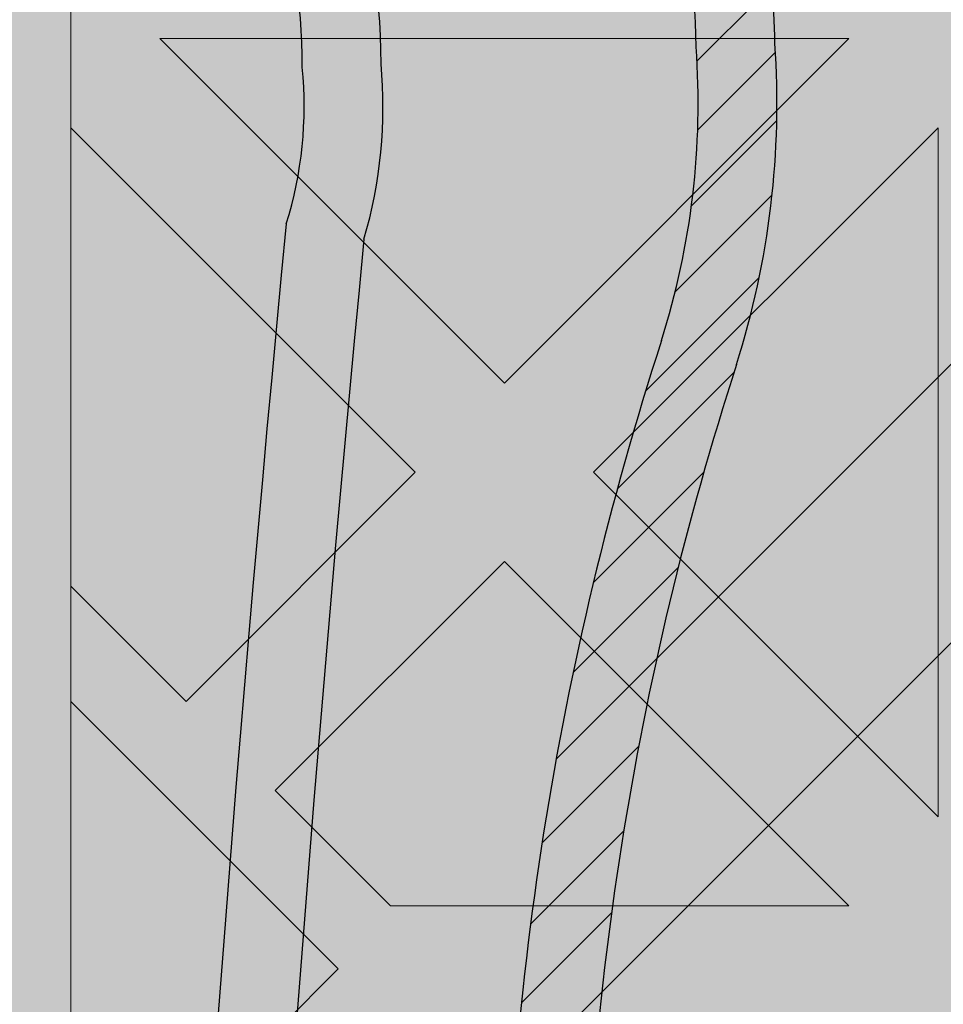
# Model space of a CAD drawing. Units: inches. Extents: x 844 to 2234, y 346 to 1084.
# Tile 17 of 93: x 1118.29 to 1120.159, y 701.25 to 703.242. Entities that reach past the tile are written whole.
import ezdxf

# ---------------------------------------------------------------- set-up
doc = ezdxf.new("R2010")
doc.units = ezdxf.units.IN
doc.header["$MEASUREMENT"] = 0
for name, color, linetype, lineweight in [('A-ANNO-DIMS', 2, 'Continuous', 18), ('furniture', 8, 'Continuous', 18), ('RA-AP-01$0$INT', 35, 'Continuous', 5)]:
    doc.layers.add(name, color=color, linetype=linetype, lineweight=lineweight)
doc.layers.add('RA-AP-01$0$FURN', color=3, linetype='Continuous')
doc.layers.add('RA-AP-01$0$WOOD', color=64, linetype='Continuous')
doc.styles.get("Standard").update_dxf_attribs({"font": 'arial.ttf'})
doc.dimstyles.get("Standard").update_dxf_attribs({"dimtxt": 6, "dimasz": 3, "dimexe": 0.18, "dimexo": 0.0625, "dimgap": 0.09, "dimtad": 0, "dimtih": 1, "dimtoh": 1, "dimdec": 1, "dimzin": 0, "dimdsep": 46, "dimlunit": 3, "dimtxsty": 'Standard', "dimblk": 'ARCHTICK', "dimcen": 0.09, "dimadec": 0, "dimazin": 0, "dimtfac": 1, "dimtdec": 1, "dimtofl": 0, "dimtmove": 0, "dimatfit": 3, "dimfxl": 1, "dimtolj": 1, "dimtzin": 0, "dimarcsym": 0})

# ---------------------------------------------------------------- blocks, each defined once
blk = doc.blocks.new('A$C18D01794')
at = {"layer": 'RA-AP-01$0$INT'}
blk.add_hatch(color=256, dxfattribs=at).paths.add_polyline_path([(4.505206456958071, -7.906712009588039), (5.305206456958072, -7.906712009588039), (5.305206456958072, -7.106712009588038), (5.255206456951893, -7.106712009588036), (5.25520645694868, -7.856712009570104), (4.555206456959269, -7.856712009588616), (4.555206456956052, -7.106712009588038), (4.505206456958073, -7.106712009588038)])
h = blk.add_hatch(color=256, dxfattribs=at)
h.paths.add_polyline_path([(4.585917135068448, -7.856712009587804), (4.614201406330596, -7.856712009587056), (4.668846067270487, -7.802067348644738), (4.723490728212344, -7.856712009584164), (4.771774999457151, -7.856712009582887), (4.826419660396886, -7.80206734864072), (4.862780050090322, -7.838427738332541), (4.844495778842715, -7.856712009580965), (4.862780050090411, -7.856712009580482), (4.905206456960182, -7.814285602707865), (4.947632863832445, -7.856712009578238), (4.965917135079675, -7.856712009577755), (4.947632863831759, -7.838427738330656), (4.983993253523576, -7.802067348637219), (5.038637914464627, -7.856712009575829), (5.08692218571208, -7.856712009574554), (5.141566846649976, -7.802067348634224), (5.196211507589851, -7.856712009571666), (5.224495778822615, -7.856712009570916), (4.905206456953975, -7.537422687702283)])
h.paths.add_polyline_path([(4.895206456956031, -7.575706958950402), (4.895206456958921, -7.684996280828174), (4.840561796018589, -7.630351619890275)], flags=16)
h.paths.add_polyline_path([(4.915206456955638, -7.575706958949956), (4.969851117895509, -7.630351619887399), (4.915206456957609, -7.684996280827732)], flags=16)
h.paths.add_polyline_path([(4.826419660395175, -7.644493755514321), (4.881064321335613, -7.699138416452331), (4.771774999456703, -7.69913841645522)], flags=16)
h.paths.add_polyline_path([(4.983993253519558, -7.644493755510815), (5.038637914460456, -7.699138416449285), (4.929348592581548, -7.69913841645126)], flags=16)
h.paths.add_polyline_path([(4.881064321336025, -7.719138416452334), (4.826419660397532, -7.773783077393256), (4.771774999457062, -7.719138416455217)], flags=16)
h.paths.add_polyline_path([(4.929348592582019, -7.71913841645126), (5.038637914460982, -7.719138416449284), (4.983993253522945, -7.773783077389749)], flags=16)
h.paths.add_polyline_path([(4.895206456960191, -7.733280552075633), (4.895206456962115, -7.806001331460164), (4.876922185715016, -7.824285602708492), (4.840561796021581, -7.787925213016675)], flags=16)
h.paths.add_polyline_path([(4.915206456958487, -7.733280552075187), (4.969851117899527, -7.787925213013798), (4.933490728206909, -7.824285602708034), (4.9152064569598, -7.806001331461736)], flags=16)
h.paths.add_polyline_path([(4.757632863832376, -7.733280552079264), (4.812277524772842, -7.787925213017304), (4.757632863834348, -7.842569873958233)], flags=16)
h.paths.add_polyline_path([(4.737632863832376, -7.73328055207979), (4.737632863834348, -7.842569873958701), (4.682988202893906, -7.787925213020692)], flags=16)
h.paths.add_polyline_path([(5.05278005008503, -7.733280552072701), (5.052780050087917, -7.842569873951664), (4.998135389146995, -7.787925213013169)], flags=16)
h.paths.add_polyline_path([(5.072780050085024, -7.733280552072333), (5.127424711025931, -7.787925213010806), (5.072780050087916, -7.842569873951244)], flags=16)
h.paths.add_polyline_path([(4.935917135072783, -7.506712009583784), (5.255206456948811, -7.826001331459767), (5.255206456948932, -7.797717060211899), (5.200561796010279, -7.743072399273238), (5.255206456949403, -7.688427738334128), (5.25520645694961, -7.640143467086677), (5.200561796009787, -7.585498806146837), (5.236922185702417, -7.549138416454212), (5.255206456949919, -7.56742268770172), (5.255206456949998, -7.549138416454178), (5.212780050078687, -7.506712009583814), (5.25520645695036, -7.464285602712145), (5.255206456950438, -7.446001331464763), (5.236922185702424, -7.464285602712779), (5.200561796009796, -7.427925213020149), (5.255206456950753, -7.373280552079203), (5.25520645695096, -7.324996280834394), (5.200561796010322, -7.270351619893748), (5.255206456951428, -7.215706958952649), (5.255206456951547, -7.187422687705071)])
h.paths.add_polyline_path([(5.042988202883395, -7.42792521302065), (5.097632863823085, -7.373280552080975), (5.097632863822622, -7.482569873959883)], flags=16)
h.paths.add_polyline_path([(5.028846067259663, -7.442067348644384), (5.083490728198774, -7.496712009583504), (4.974201406321001, -7.496712009583035)], flags=16)
h.paths.add_polyline_path([(5.117632863823087, -7.37328055208089), (5.172277524762331, -7.42792521302015), (5.11763286382262, -7.482569873959851)], flags=16)
h.paths.add_polyline_path([(5.08349072819877, -7.516712009582191), (5.028846067259652, -7.571356670521302), (4.974201406320998, -7.516712009582638)], flags=16)
h.paths.add_polyline_path([(5.131774999446817, -7.35913841645716), (5.186419660386065, -7.413783077396415), (5.241064321325782, -7.359138416456712)], flags=17)
h.paths.add_polyline_path([(5.131774999446228, -7.496712009583703), (5.186419660386065, -7.442067348643883), (5.222780050079488, -7.478427738337313), (5.204495778832781, -7.496712009584014)], flags=16)
h.paths.add_polyline_path([(5.097632863822613, -7.530854145205813), (5.097632863823061, -7.640143467084723), (5.042988202883383, -7.585498806145032)], flags=16)
h.paths.add_polyline_path([(5.131774999446899, -7.339138416457162), (5.241064321325809, -7.339138416456712), (5.186419660386591, -7.284493755517479)], flags=17)
h.paths.add_polyline_path([(5.131774999446226, -7.516712009581999), (5.204495778830767, -7.516712009581702), (5.22278005007868, -7.534996280829206), (5.186419660386049, -7.571356670521828)], flags=16)
h.paths.add_polyline_path([(5.11763286382262, -7.530854145205852), (5.17227752476232, -7.585498806145562), (5.117632863823064, -7.64014346708481)], flags=16)
h.paths.add_polyline_path([(5.186419660386069, -7.599640941770585), (5.241064321325754, -7.654285602710281), (5.131774999446791, -7.654285602709814)], flags=16)
h.paths.add_polyline_path([(5.131774999446872, -7.674285602709813), (5.24106432132578, -7.674285602710282), (5.186419660386554, -7.728930263649504)], flags=16)
h.paths.add_polyline_path([(5.255206456951811, -7.126001331467467), (5.255206456951895, -7.106712009588038), (4.555206456956052, -7.106712009588038), (4.555206456956136, -7.12600133146746), (4.905206456953973, -7.476001331465289)])
h.paths.add_polyline_path([(4.983993253513404, -7.368930263651977), (4.92934859257295, -7.314285602713969), (5.03863791445186, -7.314285602711063)], flags=16)
h.paths.add_polyline_path([(4.969851117889988, -7.383072399276016), (4.915206456952556, -7.437717060215906), (4.915206456949648, -7.328427738338133)], flags=16)
h.paths.add_polyline_path([(4.929348592572535, -7.294285602713971), (4.983993253511019, -7.239640941773039), (5.038637914451496, -7.294285602711065)], flags=16)
h.paths.add_polyline_path([(5.052780050074912, -7.280143467087016), (4.998135389134438, -7.225498806148989), (5.052780050072919, -7.170854145208052)], flags=16)
h.paths.add_polyline_path([(5.07278005007491, -7.280143467086489), (5.072780050072918, -7.170854145207579), (5.127424711013374, -7.225498806145578)], flags=16)
h.paths.add_polyline_path([(4.89520645695295, -7.437717060216355), (4.840561796013067, -7.383072399278919), (4.895206456950961, -7.328427738338582)], flags=16)
h.paths.add_polyline_path([(4.915206456948365, -7.280143467090674), (4.915206456946434, -7.207422687704125), (4.933490728192729, -7.18913841645701), (4.969851117886972, -7.225498806149623)], flags=16)
h.paths.add_polyline_path([(4.881064321327021, -7.314285602715054), (4.82641966038902, -7.368930263655506), (4.771774999448108, -7.314285602717047)], flags=16)
h.paths.add_polyline_path([(4.895206456950073, -7.280143467091125), (4.840561796009022, -7.225498806152518), (4.876922185700835, -7.18913841645908), (4.895206456948749, -7.207422687706589)], flags=16)
h.paths.add_polyline_path([(4.983993253510392, -7.211356670525576), (4.947632863816944, -7.174996280833758), (4.965917135064043, -7.156712009585847), (5.038637914448995, -7.156712009584522)], flags=16)
h.paths.add_polyline_path([(4.881064321326543, -7.294285602715056), (4.771774999447578, -7.294285602717046), (4.826419660385607, -7.239640941776569)], flags=16)
h.paths.add_polyline_path([(4.905206456946447, -7.19913841645844), (4.862780050074785, -7.156712009587725), (4.947632863816685, -7.156712009586302)], flags=16)
h.paths.add_polyline_path([(5.14156684663679, -7.211356670521528), (5.086922185696452, -7.156712009583639), (5.196211507574223, -7.156712009581651)], flags=16)
h.paths.add_polyline_path([(4.8264196603837, -7.211356670529104), (4.771774999442643, -7.156712009590501), (4.8444957788276, -7.156712009588568), (4.862780050075511, -7.17499628083566)], flags=16)
h.paths.add_polyline_path([(4.812277524760289, -7.225498806153156), (4.757632863822258, -7.28014346709363), (4.757632863819352, -7.170854145214669)], flags=16)
h.paths.add_polyline_path([(4.73763286382226, -7.280143467093997), (4.682988202881349, -7.22549880615554), (4.737632863819352, -7.170854145215086)], flags=16)
h.paths.add_polyline_path([(4.723490728195188, -7.156712009591787), (4.668846067257299, -7.211356670532127), (4.614201406317417, -7.156712009594693)], flags=16)
h.paths.add_polyline_path([(4.597632863829262, -7.506712009583814), (4.555206456957951, -7.54913841645418), (4.555206456958029, -7.56742268770172), (4.573490728205535, -7.549138416454212), (4.609851117898167, -7.585498806146839), (4.555206456958338, -7.640143467086675), (4.555206456958546, -7.688427738334125), (4.60985111789767, -7.743072399273238), (4.555206456959015, -7.797717060211899), (4.555206456959138, -7.826001331459767), (4.874495778835167, -7.506712009583786), (4.5552064569564, -7.187422687705062), (4.555206456956523, -7.215706958952644), (4.609851117897629, -7.270351619893746), (4.555206456956988, -7.324996280834396), (4.555206456957198, -7.373280552079195), (4.609851117898153, -7.427925213020147), (4.573490728205528, -7.464285602712779), (4.555206456957507, -7.446001331464756), (4.555206456957585, -7.464285602712143)])
h.paths.add_polyline_path([(4.712780050085332, -7.482569873959882), (4.712780050084863, -7.373280552080972), (4.767424711024555, -7.42792521302065)], flags=16)
h.paths.add_polyline_path([(4.726922185709173, -7.496712009583504), (4.781566846648288, -7.442067348644384), (4.836211507586949, -7.496712009583033)], flags=16)
h.paths.add_polyline_path([(4.692780050085327, -7.482569873959851), (4.638135389145619, -7.427925213020149), (4.692780050084865, -7.373280552080892)], flags=16)
h.paths.add_polyline_path([(4.726922185709182, -7.516712009582191), (4.836211507586949, -7.51671200958264), (4.7815668466483, -7.571356670521304)], flags=16)
h.paths.add_polyline_path([(4.678637914461726, -7.496712009583706), (4.605917135075169, -7.496712009584014), (4.587632863828464, -7.478427738337311), (4.623993253521887, -7.442067348643881)], flags=16)
h.paths.add_polyline_path([(4.712780050085336, -7.530854145205816), (4.767424711024568, -7.585498806145034), (4.71278005008489, -7.640143467084724)], flags=16)
h.paths.add_polyline_path([(4.678637914461726, -7.516712009582001), (4.623993253521899, -7.571356670521829), (4.587632863829271, -7.534996280829206), (4.605917135077185, -7.5167120095817)], flags=16)
h.paths.add_polyline_path([(4.692780050085336, -7.530854145205848), (4.692780050084889, -7.64014346708481), (4.638135389145632, -7.585498806145562)], flags=16)
h.paths.add_polyline_path([(4.623993253521885, -7.413783077396415), (4.678637914461131, -7.359138416457161), (4.56934859258217, -7.359138416456712)], flags=17)
h.paths.add_polyline_path([(4.623993253521901, -7.599640941770568), (4.678637914461158, -7.654285602709814), (4.569348592582195, -7.654285602710281)], flags=16)
h.paths.add_polyline_path([(4.678637914461051, -7.339138416457162), (4.623993253521361, -7.284493755517479), (4.569348592582143, -7.339138416456712)], flags=17)
h.paths.add_polyline_path([(4.678637914461076, -7.674285602709813), (4.623993253521399, -7.728930263649504), (4.569348592582167, -7.674285602710281)], flags=16)
h = blk.add_hatch(color=256, dxfattribs=at)
h.paths.add_polyline_path([(4.781566846647504, -7.442067348645805), (4.836211507586161, -7.496712009584463), (4.726922185708388, -7.496712009584918)])
h.paths.add_polyline_path([(4.836211507586161, -7.516712009584068), (4.781566846647504, -7.571356670522723), (4.726922185708388, -7.516712009583606)])
h.paths.add_polyline_path([(4.76742471102377, -7.585498806146453), (4.712780050084083, -7.640143467086137), (4.712780050084542, -7.530854145207227)])
h.paths.add_polyline_path([(4.692780050084544, -7.530854145207257), (4.692780050084084, -7.64014346708622), (4.638135389144834, -7.585498806146965)])
h.paths.add_polyline_path([(4.678637914460932, -7.516712009583407), (4.623993253521102, -7.571356670523233), (4.587632863827676, -7.53499628082981), (4.605917135074382, -7.516712009583104)])
h.paths.add_polyline_path([(4.573490728204743, -7.54913841645434), (4.60985111789737, -7.585498806146969), (4.555206456957541, -7.640143467086797), (4.555206456957237, -7.567422687701846)])
h.paths.add_polyline_path([(4.623993253521098, -7.599640941770699), (4.67863791446035, -7.654285602709951), (4.56934859258139, -7.654285602710407)])
h.paths.add_polyline_path([(4.678637914460275, -7.67428560270995), (4.623993253520583, -7.728930263649637), (4.56934859258136, -7.674285602710405)])
h.paths.add_polyline_path([(4.609851117896854, -7.743072399273369), (4.555206456958196, -7.797717060212026), (4.555206456957738, -7.688427738334254)])
h.paths.add_polyline_path([(4.597632863828475, -7.506712009583301), (4.555206456957283, -7.549138416454495), (4.555206456956805, -7.464285602712587)])
h.paths.add_polyline_path([(4.678637914460932, -7.496712009585113), (4.605917135076396, -7.496712009585417), (4.587632863828479, -7.478427738337913), (4.623993253521104, -7.442067348645284)])
h.paths.add_polyline_path([(4.692780050084091, -7.373280552082301), (4.692780050084548, -7.482569873961267), (4.638135389144834, -7.427925213021552)])
h.paths.add_polyline_path([(4.767424711023772, -7.427925213022072), (4.712780050084545, -7.48256987396129), (4.712780050084089, -7.373280552082384)])
h.paths.add_polyline_path([(4.67863791446036, -7.359138416457298), (4.623993253521105, -7.41378307739655), (4.569348592581399, -7.35913841645684)])
h.paths.add_polyline_path([(4.609851117897371, -7.427925213020278), (4.573490728204743, -7.464285602712907), (4.555206456957237, -7.446001331465401), (4.555206456957548, -7.373280552080448)])
h.paths.add_polyline_path([(4.623993253520596, -7.284493755517612), (4.67863791446028, -7.339138416457299), (4.569348592581367, -7.339138416456838)])
h.paths.add_polyline_path([(4.609851117896867, -7.270351619893878), (4.555206456957749, -7.324996280832994), (4.55520645695821, -7.21570695895522)])
for p, q in [((4.555206456956052, -7.106712009588036), (4.555206456959269, -7.856712009588616)), ((4.597632863829264, -7.506712009583814), (4.55520645695807, -7.464285602712626)), ((4.55520645695807, -7.464285602712626), (4.555206456957598, -7.549138416454534)), ((4.597632863829264, -7.506712009583814), (4.555206456957598, -7.549138416454534)), ((4.605917135074869, -7.516712009584017), (4.587632863829269, -7.534996280829206)), ((4.605917135076771, -7.5167120095817), (4.678637914461723, -7.516712009581999)), ((4.678637914461723, -7.516712009581999), (4.623993253521898, -7.571356670521829)), ((4.692780050085336, -7.530854145205847), (4.638135389145632, -7.585498806145562)), ((4.692780050084889, -7.64014346708481), (4.692780050085336, -7.530854145205847)), ((4.623993253521899, -7.571356670521829), (4.587632863829269, -7.534996280829206)), ((4.555206456958031, -7.56742268770172), (4.573490728205535, -7.549138416454212)), ((4.609851117898167, -7.585498806146839), (4.573490728205535, -7.549138416454214)), ((4.555206456958033, -7.56742268770172), (4.555206456958345, -7.640143467086671)), ((4.555206456958345, -7.640143467086671), (4.609851117898167, -7.585498806146837)), ((4.692780050084889, -7.64014346708481), (4.638135389145632, -7.585498806145562)), ((4.569348592582195, -7.654285602710281), (4.623993253521901, -7.599640941770568)), ((4.678637914461158, -7.654285602709814), (4.623993253521901, -7.599640941770568)), ((4.678637914461158, -7.654285602709814), (4.569348592582195, -7.654285602710281))]:
    blk.add_line(p, q, dxfattribs=at)
blk = doc.blocks.new('A$C32926AE1')
at = {"layer": 'RA-AP-01$0$WOOD'}
h = blk.add_hatch(color=256, dxfattribs=at)
h.dxf.hatch_style = 1
h.paths.add_polyline_path([(5.157430609644524, 4.573483066760929, -0.1009492694046607), (5.155401577623758, 4.593365984175333, -0.1842662638101597), (5.172249623284174, 4.638795604568598, 0.2056608120311276), (5.179560981299304, 4.661316324430096, 0.3614336704623542), (5.134352340494423, 4.706524965234944, 0.2056608120311297), (5.111831620632933, 4.699213607219793, -0.1842662638101113), (5.066402000239693, 4.682365561559342, -0.1055311479399994), (5.045656153913092, 4.68467289944697, 0.1567636581983829), (4.763886414745334, 4.684672899446966, -0.1055311479399895), (4.743140568418733, 4.68236556155934, -0.1842662638100833), (4.6977109480255, 4.69921360721979, 0.2056608120302612), (4.675190228164109, 4.706524965234949, 0.3614336704708441), (4.629981587358889, 4.66131632442871, 0.2056608120245944), (4.637292945374126, 4.638795604567974, -0.1842662638101024), (4.654140991034615, 4.59336598417475, -0.1009492694055169), (4.652111959013835, 4.573483066760181, 0.021410119221476), (4.629748025606143, 4.156712009541676, 0.0214101192214795), (4.652111959013809, 3.739940952323101, -0.1009492694059586), (4.654140991034615, 3.720058034908448, -0.1842662638100975), (4.637292945374126, 3.674628414515226, 0.2056608120245705), (4.629981587358889, 3.652107694654492, 0.3614336704708879), (4.675190228164113, 3.606899053848249, 0.2056608120302384), (4.697710948025501, 3.614210411863408, -0.1842662638100995), (4.743140568418738, 3.63105845752386, -0.1055311479402541), (4.763886414745388, 3.628751119636215, 0.1567636581983776), (5.045656153913137, 3.628751119636244, -0.1055311479397538), (5.066402000239692, 3.631058457523857, -0.1842662638101067), (5.111831620632931, 3.614210411863407, 0.2056608120310924), (5.134352340494417, 3.606899053848256, 0.3614336704624001), (5.179560981299307, 3.652107694653103, 0.2056608120311314), (5.172249623284175, 3.6746284145146, -0.1842662638101402), (5.155401577623758, 3.72005803490786, -0.1009492694051366), (5.15743060964455, 3.739940952322354, 0.0214101192215073), (5.179794543052287, 4.156712009541468, 0.0214101192215252)])
h.paths.add_polyline_path([(4.639748609479751, 4.156712009541513, 0.0213537860821624), (4.661970494867118, 3.741887061152232, -0.094075836301374), (4.664143710413708, 3.7196126951003, -0.1824818158568985), (4.644813765429836, 3.668037719127816, 0.2056608120245319), (4.639939526753007, 3.653023905887301, 0.3614336704710246), (4.676106439397173, 3.616856993242342, 0.2056608120302234), (4.691120252638095, 3.621731231919122, -0.1824818158602558), (4.742695228611606, 3.641061176902986, -0.1029891339458722), (4.766991894714349, 3.638256818950944, 0.156709409989566), (5.042550673941472, 3.638256818950105, -0.102989133958497), (5.066847340047078, 3.641061176902949, -0.1824818158594995), (5.118422316020358, 3.621731231919103, 0.2056608120311416), (5.133436129261316, 3.616856993242346, 0.3614336704621468), (5.169603041905217, 3.653023905886178, 0.2056608120310986), (5.164728803228477, 3.668037719127177, -0.1824818158565612), (5.145398858244737, 3.719612695099578, -0.0940758363009313), (5.147572073791232, 3.741887061151398, 0.0213537860822023), (5.169793959178681, 4.156712009541451, 0.0213537860822226), (5.147572073791203, 4.571536957931898, -0.0940758363005034), (5.145398858244737, 4.59381132398362, -0.1824818158565587), (5.164728803228476, 4.645386299956021, 0.2056608120311045), (5.169603041905216, 4.66040011319702, 0.3614336704621845), (5.133436129261313, 4.696567025840856, 0.2056608120310773), (5.118422316020359, 4.691692787164098, -0.182481815859508), (5.066847340047078, 4.67236284218025, -0.1029891339584606), (5.04255067394148, 4.675167200133092, 0.156709409989566), (4.766991894714357, 4.675167200132257, -0.1029891339458842), (4.742695228611611, 4.672362842180213, -0.1824818158602725), (4.691120252638095, 4.691692787164077, 0.2056608120302152), (4.676106439397174, 4.696567025840858, 0.3614336704710363), (4.639939526753005, 4.660400113195899, 0.2056608120245495), (4.644813765429837, 4.645386299955384, -0.1824818158568934), (4.664143710413708, 4.593811323982902, -0.0940758363009187), (4.661970494867149, 4.571536957931074, 0.021353786082177)], flags=16)
h.paths.add_polyline_path([(5.129794543052235, 4.432167055276933, -0.0141661062790638), (5.130152669293814, 4.156927903047693, -0.0141661062790647), (5.129794543052234, 3.881688750818433, -0.0785247771143638), (5.10979738006795, 3.755143611847103, 0.0945969212073497), (5.105408519571111, 3.717898134952927, 0.1043170707844957), (5.116074640131521, 3.670385395016088, 0.1043170707864965), (5.068561900193738, 3.681051515576561, 0.09459692119553), (5.031316423304057, 3.676662655080835, -0.1580239521427272), (4.778226145355827, 3.676662655080367, 0.0945969211986668), (4.740980668464973, 3.681051515576592, 0.1043170707882822), (4.693467928526415, 3.670385395015844, 0.1043170707867916), (4.704134049087309, 3.717898134953662, 0.0945969211972894), (4.69974518859162, 3.755143611844042, -0.0785247771163196), (4.679748025606343, 3.881688750818406, -0.0141661062790663), (4.679389899364763, 4.156927903047693, -0.0141661062790672), (4.679748025606343, 4.432167055276998, -0.0785247771163064), (4.699745188591625, 4.55871219425134, 0.094596921197333), (4.704134049087308, 4.595957671141738, 0.1043170707867205), (4.693467928526416, 4.643470411079523, 0.1043170707882628), (4.740980668464965, 4.632804290518776, 0.0945969211988114), (4.778226145355874, 4.637193151015016, -0.158023952142669), (5.031316423304015, 4.637193151014546, 0.0945969211956361), (5.068561900193736, 4.632804290518806, 0.1043170707864979), (5.11607464013152, 4.643470411079278, 0.1043170707844617), (5.105408519571112, 4.595957671142455, 0.0945969212074597), (5.109797380067959, 4.558712194248236, -0.0785247771143467)], flags=0)
h.paths.add_polyline_path([(5.119794532311105, 4.432259799204851, -0.0142000800617244), (5.120156169157484, 4.156927903047701, -0.0142000800617277), (5.119794532311105, 3.881596006890482, -0.0784894509520253), (5.100273383573699, 3.758192358677797, 0.0940138827242913), (5.095413455884425, 3.717477693979438, 0.0606271852308753), (5.099615656341024, 3.686844378806616, 0.0606271852322524), (5.068982341167493, 3.691046579263239, 0.0940138827010453), (5.028267676478798, 3.686186651576848, -0.1580706864508061), (4.781274892180912, 3.686186651576435, 0.0940138827026903), (4.740560227491556, 3.691046579263279, 0.0606271852339895), (4.709926912317155, 3.686844378806508, 0.0606271852329405), (4.714129112773991, 3.717477693980356, 0.094013882701304), (4.709269185087677, 3.758192358669163, -0.0784894509577193), (4.689748036347473, 3.881596006890469, -0.014200080061729), (4.689386399501094, 4.156927903047709, -0.0142000800617217), (4.689748036347473, 4.432259799204808, -0.078489450957724), (4.709269185087651, 4.555663447426125, 0.0940138827014585), (4.714129112773992, 4.596378112114996, 0.0606271852329731), (4.709926912317154, 4.62701142728886, 0.0606271852340196), (4.74056022749157, 4.622809226832087, 0.0940138827024997), (4.781274892180847, 4.627669154518912, -0.1580706864508359), (5.028267676478777, 4.627669154518526, 0.0940138827010946), (5.068982341167492, 4.622809226832129, 0.060627185232254), (5.099615656341024, 4.627011427288751, 0.0606271852308727), (5.095413455884425, 4.59637811211593, 0.0940138827241088), (5.100273383573675, 4.555663447417647, -0.0784894509520978)], flags=0)
h.paths.add_polyline_path([(5.06978912287499, 4.430218106756144, -0.014241683694547), (5.070173729147532, 4.156927903047672, -0.0142416836945458), (5.06978912287499, 3.883637699339223, -0.0800609523125196), (5.052662118612511, 3.773463122773442, 0.0526421978001116), (5.04590916754064, 3.740550867606997, 0.0526421977992423), (5.012996912374707, 3.73379791653534, -0.1583028414718258), (4.796545656286308, 3.73379791653451, 0.0526421978034211), (4.763633401117837, 3.740550867607021, 0.0526421978018622), (4.756880450045755, 3.773463122774558, -0.0800609523117106), (4.739753445783639, 3.883637699339268, -0.0142416836945435), (4.739368839511098, 4.156927903047671, -0.0142416836945477), (4.739753445783639, 4.430218106756155, -0.0800609523116345), (4.75688045004574, 4.540392683320762, 0.052642197801941), (4.763633401117837, 4.573304938488346, 0.0526421978035071), (4.796545656286361, 4.580057889560873, -0.1583028414717561), (5.012996912374669, 4.580057889560039, 0.0526421977993048), (5.04590916754064, 4.57330493848837, 0.0526421978002057), (5.052662118612529, 4.540392683321868, -0.080060952312477)], flags=0)
h.paths.add_polyline_path([(5.049789715110557, 4.43038092723357, -0.0143097550741839), (5.05018085590259, 4.156927903047715, -0.0143097550741854), (5.049789715110558, 3.883474878861827, -0.0800685599149176), (5.03362098255317, 3.779581877367999, 0.0306258898956367), (5.028241146483733, 3.758218888663947, 0.0306258898977031), (5.006878157778253, 3.75283905259408, -0.1583983521624096), (4.802664410878162, 3.752839052594731, 0.0306258898946014), (4.781301422174808, 3.758218888663924, 0.0306258898967912), (4.775921586105202, 3.779581877368794, -0.080068559914251), (4.759752853548071, 3.883474878861786, -0.0143097550741854), (4.759361712756037, 4.156927903047671, -0.0143097550741854), (4.759752853548071, 4.430380927233557, -0.0800685599142479), (4.775921586105193, 4.534273928726546, 0.0306258898968306), (4.781301422174808, 4.555636917431444, 0.0306258898945754), (4.802664410878143, 4.561016753500631, -0.1583983521624168), (5.006878157778244, 4.561016753501291, 0.0306258898977177), (5.028241146483733, 4.555636917431421, 0.0306258898958182), (5.03362098255321, 4.534273928727244, -0.080068559914796)], flags=0)
h.paths.add_polyline_path([(4.999766070382627, 4.428171244713864, -0.0143443147609634), (5.000198441819402, 4.156927903047689, -0.0143443147609612), (4.999766070382627, 3.885684561381556, -0.0784641635803329), (4.987356730658798, 3.799103304488872, -0.1506053783831347), (4.822185837999821, 3.79910330448882, -0.0784641635803318), (4.809776498276007, 3.885684561381509, -0.014344314760963), (4.809344126839227, 4.156927903047677, -0.0143443147609645), (4.809776498276007, 4.428171244713873, -0.0784641635803192), (4.822185837999822, 4.514752501606549, -0.1506053783831338), (4.987356730658798, 4.514752501606494, -0.078464163580285)], flags=0)
h.paths.add_polyline_path([(4.979755254238824, 4.42764379880488, -0.0143772539198268), (4.980205517789977, 4.156927903047693, -0.0143772539198275), (4.979755254238824, 3.886212007290489, -0.0689242507424422), (4.971183264704897, 3.815276770442801, -0.1296645318904179), (4.838359303953726, 3.815276770442746, -0.0689242507424186), (4.829787314419809, 3.886212007290419, -0.0143772539198292), (4.829337050868653, 4.156927903047653, -0.0143772539198325), (4.829787314419809, 4.427643798804946, -0.0689242507424211), (4.838359303953725, 4.498579035652621, -0.1296645318904187), (4.971183264704897, 4.498579035652565, -0.0689242507424401)], flags=0)
h = blk.add_hatch(color=256, dxfattribs=at)
h.dxf.hatch_style = 1
h.paths.add_polyline_path([(5.145398858244737, 4.59381132398362, -0.1824818158565616), (5.164728803228476, 4.645386299956021, 0.2056608120311045), (5.169603041905216, 4.66040011319702, 0.3614336704621845), (5.133436129261313, 4.696567025840856, 0.2056608120310773), (5.118422316020359, 4.691692787164098, -0.182481815859508), (5.066847340047078, 4.67236284218025, -0.1029891339584606), (5.04255067394148, 4.675167200133092, 0.156709409989566), (4.766991894714357, 4.675167200132257, -0.1029891339458842), (4.742695228611611, 4.672362842180213, -0.1824818158602725), (4.691120252638095, 4.691692787164077, 0.2056608120302152), (4.676106439397174, 4.696567025840858, 0.3614336704710363), (4.639939526753005, 4.660400113195899, 0.2056608120245495), (4.644813765429837, 4.645386299955384, -0.1824818158568934), (4.664143710413708, 4.593811323982902, -0.0940758363009187), (4.661970494867149, 4.571536957931074, 0.0213537860821772), (4.639748609479751, 4.156712009541507, 0.0213537860821625), (4.661970494867119, 3.741887061152226, -0.0940758363013071), (4.664143710413708, 3.719612695100309, -0.1824818158569294), (4.644813765429836, 3.668037719127816, 0.2056608120245319), (4.639939526753007, 3.653023905887301, 0.3614336704710246), (4.676106439397173, 3.616856993242342, 0.2056608120302234), (4.691120252638095, 3.621731231919122, -0.1824818158602558), (4.742695228611606, 3.641061176902986, -0.1029891339458722), (4.766991894714349, 3.638256818950944, 0.156709409989566), (5.042550673941472, 3.638256818950105, -0.102989133958497), (5.066847340047078, 3.641061176902949, -0.1824818158594995), (5.118422316020358, 3.621731231919103, 0.2056608120311416), (5.133436129261316, 3.616856993242346, 0.3614336704621468), (5.169603041905217, 3.653023905886178, 0.2056608120310986), (5.164728803228477, 3.668037719127177, -0.1824818158565612), (5.145398858244737, 3.719612695099578, -0.0940758363009313), (5.147572073791232, 3.741887061151398, 0.0213537860822023), (5.169793959178681, 4.156712009541451, 0.0213537860822226), (5.147572073791203, 4.571536957931898, -0.0940758363004996)])
h.paths.add_polyline_path([(5.109797380067958, 4.55871219424824, -0.0785247771143472), (5.129794543052234, 4.432167055276936, -0.0141661062790644), (5.130152669293814, 4.156927903047685, -0.014166106279066), (5.129794543052234, 3.881688750818401, -0.0785247771143517), (5.109797380067946, 3.755143611847092, 0.0945969212073132), (5.105408519571111, 3.717898134952929, 0.1043170707844995), (5.116074640131521, 3.670385395016088, 0.1043170707864965), (5.068561900193738, 3.681051515576561, 0.09459692119553), (5.031316423304057, 3.676662655080835, -0.1580239521427272), (4.778226145355827, 3.676662655080367, 0.0945969211986668), (4.740980668464973, 3.681051515576592, 0.1043170707882822), (4.693467928526415, 3.670385395015844, 0.1043170707867916), (4.704134049087309, 3.717898134953662, 0.0945969211972894), (4.69974518859162, 3.755143611844042, -0.0785247771163196), (4.679748025606343, 3.881688750818406, -0.0141661062790663), (4.679389899364763, 4.156927903047693, -0.0141661062790672), (4.679748025606343, 4.432167055276998, -0.0785247771163064), (4.699745188591625, 4.55871219425134, 0.094596921197333), (4.704134049087308, 4.595957671141738, 0.1043170707867205), (4.693467928526416, 4.643470411079523, 0.1043170707882628), (4.740980668464965, 4.632804290518776, 0.0945969211988114), (4.778226145355874, 4.637193151015016, -0.158023952142669), (5.031316423304015, 4.637193151014546, 0.0945969211956361), (5.068561900193736, 4.632804290518806, 0.1043170707864979), (5.11607464013152, 4.643470411079278, 0.1043170707844617), (5.105408519571112, 4.595957671142455, 0.0945969212074504)], flags=16)
h.paths.add_polyline_path([(5.100273383573655, 4.55566344741771, -0.0784894509521388), (5.119794532311105, 4.432259799204852, -0.0142000800617252), (5.120156169157484, 4.156927903047686, -0.014200080061726), (5.119794532311105, 3.881596006890502, -0.0784894509520446), (5.100273383573696, 3.758192358677786, 0.0940138827242721), (5.095413455884425, 3.717477693979436, 0.0606271852308692), (5.099615656341024, 3.686844378806616, 0.0606271852322522), (5.068982341167493, 3.691046579263239, 0.0940138827010453), (5.028267676478798, 3.686186651576848, -0.1580706864508061), (4.781274892180912, 3.686186651576435, 0.0940138827026903), (4.740560227491556, 3.691046579263279, 0.0606271852339895), (4.709926912317155, 3.686844378806508, 0.0606271852329405), (4.714129112773991, 3.717477693980356, 0.094013882701304), (4.709269185087677, 3.758192358669163, -0.0784894509577193), (4.689748036347473, 3.881596006890469, -0.014200080061729), (4.689386399501094, 4.156927903047709, -0.0142000800617217), (4.689748036347473, 4.432259799204808, -0.078489450957724), (4.709269185087651, 4.555663447426125, 0.0940138827014585), (4.714129112773992, 4.596378112114996, 0.0606271852329731), (4.709926912317154, 4.62701142728886, 0.0606271852340196), (4.74056022749157, 4.622809226832087, 0.0940138827024997), (4.781274892180847, 4.627669154518912, -0.1580706864508359), (5.028267676478777, 4.627669154518526, 0.0940138827010946), (5.068982341167492, 4.622809226832129, 0.060627185232254), (5.099615656341024, 4.627011427288751, 0.0606271852308727), (5.095413455884425, 4.59637811211593, 0.094013882723957)], flags=0)
h.paths.add_polyline_path([(5.04590916754064, 4.57330493848837, 0.0526421978002057), (5.052662118612529, 4.540392683321868, -0.0800609523124783), (5.06978912287499, 4.430218106756142, -0.0142416836945469), (5.070173729147532, 4.156927903047672, -0.0142416836945458), (5.06978912287499, 3.883637699339223, -0.0800609523125196), (5.052662118612511, 3.773463122773442, 0.0526421978001116), (5.04590916754064, 3.740550867606997, 0.0526421977992423), (5.012996912374707, 3.73379791653534, -0.1583028414718258), (4.796545656286308, 3.73379791653451, 0.0526421978034211), (4.763633401117837, 3.740550867607021, 0.0526421978018622), (4.756880450045755, 3.773463122774558, -0.0800609523117106), (4.739753445783639, 3.883637699339268, -0.0142416836945435), (4.739368839511098, 4.156927903047671, -0.0142416836945477), (4.739753445783639, 4.430218106756155, -0.0800609523116345), (4.75688045004574, 4.540392683320762, 0.052642197801941), (4.763633401117837, 4.573304938488346, 0.0526421978035071), (4.796545656286361, 4.580057889560873, -0.1583028414717561), (5.012996912374669, 4.580057889560039, 0.0526421977993048)], flags=0)
h.paths.add_polyline_path([(5.028241146483733, 4.555636917431422, 0.0306258898956949), (5.033620982553182, 4.534273928727329, -0.0800685599148649), (5.049789715110557, 4.430380927233569, -0.0143097550741839), (5.05018085590259, 4.156927903047715, -0.0143097550741854), (5.049789715110558, 3.883474878861827, -0.0800685599149176), (5.03362098255317, 3.779581877367999, 0.0306258898956367), (5.028241146483733, 3.758218888663947, 0.0306258898977031), (5.006878157778253, 3.75283905259408, -0.1583983521624096), (4.802664410878162, 3.752839052594731, 0.0306258898946014), (4.781301422174808, 3.758218888663924, 0.0306258898967912), (4.775921586105202, 3.779581877368794, -0.080068559914251), (4.759752853548071, 3.883474878861786, -0.0143097550741854), (4.759361712756037, 4.156927903047671, -0.0143097550741854), (4.759752853548071, 4.430380927233557, -0.0800685599142479), (4.775921586105193, 4.534273928726546, 0.0306258898968306), (4.781301422174808, 4.555636917431444, 0.0306258898945754), (4.802664410878143, 4.561016753500631, -0.1583983521624168), (5.006878157778244, 4.561016753501291, 0.0306258898977174)], flags=0)
h.paths.add_polyline_path([(4.987356730658798, 4.514752501606494, -0.0784641635803018), (4.999766070382627, 4.428171244713845, -0.0143443147609637), (5.000198441819402, 4.156927903047665, -0.0143443147609622), (4.999766070382628, 3.885684561381514, -0.0784641635802952), (4.987356730658797, 3.799103304488872, -0.1506053783831338), (4.822185837999821, 3.799103304488819, -0.0784641635803342), (4.809776498276007, 3.885684561381512, -0.0143443147609628), (4.809344126839227, 4.156927903047676, -0.0143443147609646), (4.809776498276007, 4.428171244713873, -0.0784641635803192), (4.822185837999822, 4.514752501606549, -0.1506053783831338)], flags=0)
h.paths.add_polyline_path([(4.971183264704897, 4.498579035652566, -0.0689242507424384), (4.979755254238824, 4.427643798804883, -0.0143772539198276), (4.980205517789977, 4.15692790304768, -0.0143772539198258), (4.979755254238823, 3.88621200729051, -0.0689242507424628), (4.971183264704897, 3.815276770442801, -0.129664531890417), (4.838359303953726, 3.815276770442746, -0.0689242507424186), (4.829787314419809, 3.886212007290419, -0.0143772539198292), (4.829337050868653, 4.156927903047653, -0.0143772539198325), (4.829787314419809, 4.427643798804946, -0.0689242507424211), (4.838359303953725, 4.498579035652621, -0.1296645318904187)], flags=0)
h = blk.add_hatch(dxfattribs=at)
h.set_pattern_fill('ANSI31', color=256, scale=0.05, style=0)
h.set_pattern_definition([(45, (0, 0), (-0.0044194173824159, 0.0044194173824159), [])])
h.paths.add_polyline_path([(5.130152669293814, 4.156927903047704, 0.0141661062790657), (5.129794543052234, 4.432167055276982, 0.0777827904001433), (5.110168979996553, 4.557559993161921, -0.0976515123401879), (5.105408519571111, 4.595957671142454, -0.1043170707844687), (5.116074640131522, 4.64347041107928), (5.099615656341024, 4.627011427288751, 0.0606271852308727), (5.095413455884425, 4.59637811211593, 0.0940138827241088), (5.100273383573675, 4.555663447417647, -0.0784894509520972), (5.119794532311105, 4.432259799204852, -0.0142000800617252), (5.120156169157484, 4.156927903047686, -0.014200080061726), (5.119794532311105, 3.881596006890502, -0.0784894509520446), (5.100273383573696, 3.758192358677786, 0.0940138827242721), (5.095413455884425, 3.717477693979436, 0.0606271852308692), (5.099615656341024, 3.686844378806616), (5.116074640131519, 3.67038539501609, -0.1043170707844594), (5.105408519571112, 3.717898134952912, -0.0976515123401594), (5.11016897999655, 3.756295812933435, 0.0777827904001654), (5.129794543052234, 3.881688750818409, 0.0141661062790665)])
h.paths.add_polyline_path([(5.030164222210597, 3.676291055149937, -0.0976515123472002), (5.068561900193739, 3.681051515576561, -0.1043170707864927), (5.116074640131521, 3.670385395016088), (5.099615656341024, 3.686844378806616, 0.0606271852322522), (5.068982341167493, 3.691046579263239, 0.0940138827010453), (5.028267676478798, 3.686186651576848, -0.1580706864508061), (4.781274892180912, 3.686186651576435, 0.0940138827026903), (4.740560227491556, 3.691046579263279, 0.0606271852339913), (4.709926912317154, 3.686844378806508), (4.693467928526416, 3.670385395015845, -0.1043170707882796), (4.740980668464973, 3.681051515576592, -0.0976515123427246), (4.779378346446416, 3.676291055150394, 0.156512506893803)])
h.paths.add_polyline_path([(4.689748036347473, 3.881596006890472, -0.014200080061729), (4.689386399501094, 4.156927903047712, -0.0142000800617195), (4.689748036347473, 4.432259799204768, -0.078489450957742), (4.709269185087648, 4.555663447426114, 0.0940138827014821), (4.714129112773992, 4.596378112114995, 0.0606271852329748), (4.709926912317154, 4.62701142728886), (4.693467928526414, 4.643470411079524, -0.1043170707867939), (4.704134049087309, 4.595957671141706, -0.09765151234893), (4.699373588660725, 4.557559993157876, 0.0777827903975372), (4.679748025606343, 4.432167055276987, 0.0141661062790675), (4.679389899364763, 4.156927903047675, 0.0141661062790641), (4.679748025606343, 3.88168875081843, 0.0777827903975637), (4.699373588660724, 3.756295812937497, -0.0976515123490278), (4.704134049087308, 3.717898134953629, -0.1043170707867196), (4.693467928526416, 3.670385395015845), (4.709926912317155, 3.686844378806508, 0.0606271852329413), (4.714129112773991, 3.717477693980357, 0.0940138827013084), (4.709269185087676, 3.758192358669166, -0.0784894509577192)])
h.paths.add_polyline_path([(4.779378346446434, 4.63756475094498, -0.0976515123427943), (4.740980668464964, 4.632804290518776, -0.1043170707882609), (4.693467928526416, 4.643470411079523), (4.709926912317154, 4.62701142728886, 0.0606271852340196), (4.74056022749157, 4.622809226832087, 0.0940138827024997), (4.781274892180847, 4.627669154518912, -0.1580706864508359), (5.028267676478777, 4.627669154518526, 0.0940138827010946), (5.068982341167492, 4.622809226832129, 0.060627185232254), (5.099615656341024, 4.627011427288751), (5.116074640131521, 4.643470411079279, -0.1043170707865022), (5.068561900193735, 4.632804290518806, -0.0976515123475899), (5.030164222210446, 4.637564750945479, 0.1565125068936924)])
h = blk.add_hatch(dxfattribs=at)
h.set_pattern_fill('ANSI32', color=256, scale=0.2, style=0)
h.set_pattern_definition([(45, (0, 0), (-0.0530330085889911, 0.0530330085889911), []), (45, (0.035355339, 0), (-0.0530330085889911, 0.0530330085889911), [])])
h.paths.add_polyline_path([(5.119794532311105, 4.432259799204823, 0.0777015974868765), (5.10065834347252, 4.554469821747928, -0.0968902511992216), (5.095413455884425, 4.596378112115931, -0.060627185230871), (5.099615656341024, 4.627011427288751, -0.060627185232254), (5.068982341167492, 4.622809226832129, -0.0968902512198245), (5.027074050790956, 4.628054114423209, 0.1564657949319105), (4.782468517866163, 4.628054114422785, -0.0968902512152247), (4.740560227491555, 4.622809226832088, -0.0606271852339878), (4.709926912317155, 4.627011427288859, -0.0606271852329413), (4.714129112773991, 4.596378112115011, -0.0968902512205338), (4.708884225182929, 4.554469821738175, 0.0777015974804443), (4.689748036347473, 4.43225979920482, 0.0142000800617215), (4.689386399501094, 4.156927903047726, 0.0142000800617273), (4.689748036347473, 3.88159600689052, 0.077701597480541), (4.708884225182985, 3.759385984357019, -0.096890251220082), (4.714129112773992, 3.717477693980371, -0.0606271852329731), (4.709926912317154, 3.686844378806507, -0.060627185233988), (4.740560227491554, 3.691046579263279, -0.0968902512152569), (4.782468517866175, 3.685801691672578, 0.1564657949319236), (5.027074050790988, 3.685801691672169, -0.0968902512197451), (5.068982341167491, 3.691046579263239, -0.0606271852322557), (5.099615656341024, 3.686844378806616, -0.0606271852308727), (5.095413455884425, 3.717477693979438, -0.0968902511991229), (5.100658343472507, 3.7593859843474, 0.0777015974868745), (5.119794532311105, 3.8815960068905, 0.014200080061726), (5.120156169157484, 4.156927903047685, 0.0142000800617238)])
h.paths.add_polyline_path([(5.070173729147531, 4.156927903047684, -0.0142416836945481), (5.06978912287499, 3.883637699339191, -0.0800609523125107), (5.052662118612505, 3.773463122773424, 0.0526421978000811), (5.04590916754064, 3.740550867606997, 0.0526421977993214), (5.012996912374658, 3.733797916535325, -0.1583028414717916), (4.796545656286304, 3.733797916534512, 0.0526421978034138), (4.763633401117837, 3.740550867607021, 0.0526421978018622), (4.756880450045755, 3.773463122774558, -0.0800609523117106), (4.739753445783639, 3.883637699339268, -0.0142416836945435), (4.739368839511098, 4.156927903047671, -0.0142416836945477), (4.739753445783639, 4.430218106756155, -0.0800609523116345), (4.75688045004574, 4.540392683320762, 0.052642197801941), (4.763633401117837, 4.573304938488346, 0.0526421978035071), (4.796545656286361, 4.580057889560873, -0.1583028414717561), (5.012996912374669, 4.580057889560039, 0.0526421977993048), (5.04590916754064, 4.57330493848837, 0.0526421978002057), (5.052662118612529, 4.540392683321868, -0.0800609523124783), (5.06978912287499, 4.430218106756142, -0.0142416836945463)], flags=16)
h.paths.add_polyline_path([(5.050180855902591, 4.156927903047686, -0.0143097550741856), (5.049789715110558, 3.883474878861795, -0.0800685599148126), (5.033620982553202, 3.7795818773681, 0.0306258898957837), (5.028241146483733, 3.758218888663947, 0.0306258898977031), (5.006878157778253, 3.75283905259408, -0.1583983521624096), (4.802664410878162, 3.752839052594731, 0.0306258898946014), (4.781301422174808, 3.758218888663924, 0.0306258898967912), (4.775921586105202, 3.779581877368794, -0.080068559914251), (4.759752853548071, 3.883474878861786, -0.0143097550741854), (4.759361712756037, 4.156927903047671, -0.0143097550741854), (4.759752853548071, 4.430380927233557, -0.0800685599142479), (4.775921586105193, 4.534273928726546, 0.0306258898968306), (4.781301422174808, 4.555636917431444, 0.0306258898945754), (4.802664410878143, 4.561016753500631, -0.1583983521624168), (5.006878157778244, 4.561016753501291, 0.0306258898977177), (5.028241146483733, 4.555636917431421, 0.0306258898958182), (5.03362098255321, 4.534273928727244, -0.0800685599147973), (5.049789715110557, 4.430380927233568, -0.0143097550741854)], flags=0)
h.paths.add_polyline_path([(5.000198441819402, 4.15692790304769, -0.0143443147609622), (4.999766070382627, 3.885684561381539, -0.0784641635803169), (4.987356730658798, 3.799103304488873, -0.1506053783831347), (4.822185837999821, 3.79910330448882, -0.0784641635803318), (4.809776498276007, 3.885684561381509, -0.014344314760963), (4.809344126839227, 4.156927903047677, -0.0143443147609645), (4.809776498276007, 4.428171244713873, -0.0784641635803192), (4.822185837999822, 4.514752501606549, -0.1506053783831338), (4.987356730658798, 4.514752501606494, -0.0784641635803018), (4.999766070382627, 4.428171244713845, -0.0143443147609624)], flags=0)
h.paths.add_polyline_path([(4.980205517789976, 4.156927903047707, -0.0143772539198295), (4.979755254238824, 3.886212007290466, -0.06892425074242), (4.971183264704897, 3.815276770442801, -0.129664531890417), (4.838359303953726, 3.815276770442746, -0.0689242507424186), (4.829787314419809, 3.886212007290419, -0.0143772539198292), (4.829337050868653, 4.156927903047653, -0.0143772539198325), (4.829787314419809, 4.427643798804946, -0.0689242507424211), (4.838359303953725, 4.498579035652621, -0.1296645318904187), (4.971183264704897, 4.498579035652565, -0.0689242507424418), (4.979755254238824, 4.427643798804878, -0.0143772539198259)], flags=0)
for centre, radius, start, end in [((4.586173919450017, 4.593998637498934), 0.077970015963029, 359.8623536996133, 41.22894907969008), ((4.586173919450015, 4.5944304245111), 0.1179700159630316, 0.7417751874182703, 24.56332695026347), ((4.586173919450019, 4.593998637498935), 0.0679700159630267, 359.4666929486785, 41.22894907969187), ((4.586173919450018, 4.594430424511101), 0.1279700159630281, 0.8720682535796656, 14.74980897308237), ((4.604388392048173, 4.588829985554312), 0.1099999999999923, 342.4514408378524, 3.934690089293226), ((4.604388392048166, 4.588829985554355), 0.1000000000000129, 342.4716349543535, 4.087328884225124), ((4.604388392048149, 4.588398198542093), 0.0500000000000008, 342.6443160247905, 5.702070765404379), ((4.604388392048171, 4.58839819854224), 0.060000000000024, 343.6788686696151, 5.176192161067998), ((9.505218788282013, 4.104079819130551), 4.875754844654793, 174.47541031816, 179.3814986516462), ((9.505218788282013, 4.104079819130551), 4.865754844654794, 174.4870438419329, 179.3814986516462), ((5.090145208887515, 4.432167055276791), 0.4103971832811724, 162.0403002448777, 179.9999999999736), ((5.090145208887515, 4.432167055276791), 0.4003971832811724, 162.0403002448777, 179.9999999999736)]:
    blk.add_arc(centre, radius, start, end, dxfattribs=at)
blk = doc.blocks.new('A$C5D2F253E')
at = {"layer": 'RA-AP-01$0$FURN', "xscale": -0.7999999999883585, "yscale": 0.7999999999883585, "zscale": 0.8, "rotation": 90}
blk.add_blockref('A$C18D01794', (-5.687757199772477, 4.75791982714071), dxfattribs=at)
at = {"layer": 'RA-AP-01$0$WOOD', "rotation": 270}
blk.add_blockref('A$C32926AE1', (-4.161339601644158, 5.73852594588169), dxfattribs=at)
blk = doc.blocks.new('_ArchTick')
at = {"color": 0, "linetype": 'ByBlock', "const_width": 0.15}
blk.add_lwpolyline([(-0.5, -0.5), (0.5, 0.5)], dxfattribs=at)
blk = doc.blocks.new('*D144')
at = {"layer": 'A-ANNO-DIMS', "color": 0, "lineweight": -2, "transparency": 16777216}
for p, q in [((1096.615948, 439.3732739999999), (1096.615948, 1074.743301)), ((1143.115948, 492.373274), (1143.115948, 1074.743301)), ((1096.615948, 1074.563301), (1102.481950728513, 1074.563301)), ((1143.115948, 1074.563301), (1137.249945271487, 1074.563301))]:
    blk.add_line(p, q, dxfattribs=at)
at = {"layer": 'Defpoints', "color": 0, "transparency": 16777216}
for p in [(1143.115948, 1074.563301), (1143.115948, 492.3107739999999), (1096.615948, 439.3107739999999)]:
    blk.add_point(p, dxfattribs=at)
at = {"layer": 'A-ANNO-DIMS', "color": 0, "lineweight": -2, "transparency": 16777216, "xscale": 3, "yscale": 3, "zscale": 3, "rotation": 180}
blk.add_blockref('_ArchTick', (1096.615948, 1074.563301), dxfattribs=at)
at = {"layer": 'A-ANNO-DIMS', "color": 0, "lineweight": -2, "transparency": 16777216, "xscale": 3, "yscale": 3, "zscale": 3}
blk.add_blockref('_ArchTick', (1143.115948, 1074.563301), dxfattribs=at)
at = {"layer": 'A-ANNO-DIMS', "color": 0, "transparency": 16777216, "insert": (1119.865948, 1074.563301), "char_height": 6, "attachment_point": 5}
blk.add_mtext('\\A1;3\'-10 1/2"', dxfattribs=at)

msp = doc.modelspace()

# ---------------------------------------------------------------- block references
at = {"layer": 'furniture', "xscale": 15.94108302203742, "yscale": 15.94108302203742, "zscale": 15.94108302203742, "rotation": 90}
msp.add_blockref('A$C5D2F253E', (1136.147844094663, 696.2584716700112), dxfattribs=at)

# ---------------------------------------------------------------- dimensions: what is measured, and where the dimension line sits
at = {"layer": 'A-ANNO-DIMS'}
dim = msp.add_linear_dim(base=(1143.115948, 1074.563301), p1=(1096.615948, 439.3107739999999), p2=(1143.115948, 492.3107739999999), dimstyle='Standard', override={"dimdec": 1, "dimlfac": 1, "dimrnd": 0, "dimzin": 1, "dimdsep": 46, "dimlunit": 4, "dimfrac": 2}, dxfattribs=at)
dim.commit()
dim.dimension.update_dxf_attribs({"geometry": '*D144', "text_midpoint": (1119.865948, 1074.563301)})

doc.saveas('drawing.dxf')
